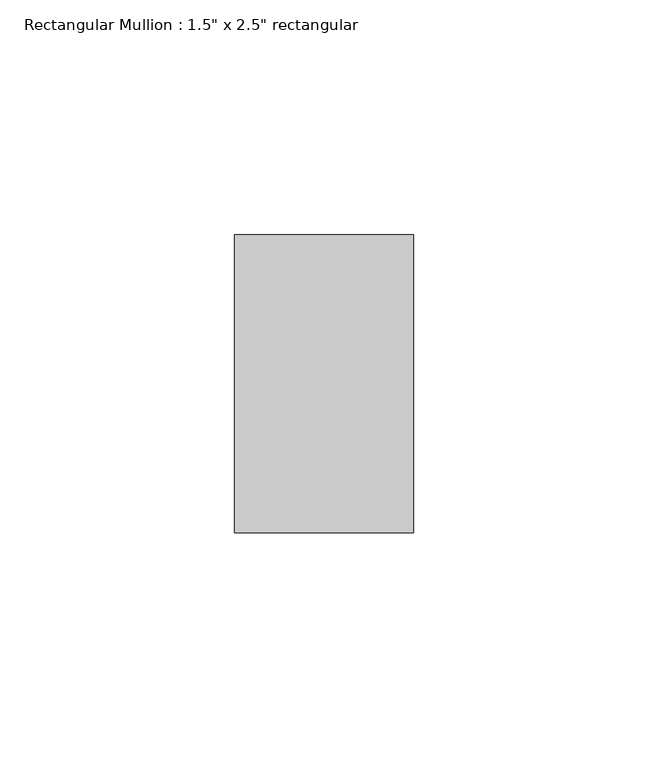
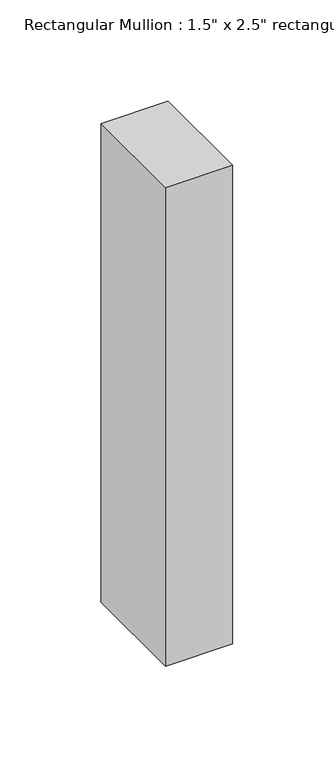
"""IFC4 building model written with IfcOpenShell, lengths in millimetres: member geometry."""

from ifc_helpers import new_model, si_unit, frame, origin, place, context, project, spatial, polyline, outline, extrude, source, transform, mapped, element, save


def member_00eacae2(model_context):
    return source(origin(), model_context, "Body", "SweptSolid", [
        extrude(outline(polyline([(19.05, 31.75), (19.05, -31.75), (-19.05, -31.75), (-19.05, 31.75), (19.05, 31.75)])), frame((0.0, 0.0, -288.2320668), z_axis=(0.0, 0.0, 1.0), x_axis=(1.0, 0.0, 0.0)), (0.0, 0.0, 1.0), 288.2320668),
    ])


if __name__ == "__main__":
    model = new_model("IFC4")
    model_context = context("Model", 3, world=origin())
    ifc_project = project(units=[si_unit("LENGTHUNIT", "METRE", prefix="MILLI")], contexts=[model_context])
    site = spatial("IfcSite", under=ifc_project)
    building = spatial("IfcBuilding", under=site)
    placement = place(None, origin())
    member_shape = member_00eacae2(model_context)
    element("IfcMember", 1, ObjectType="Rectangular Mullion : 1.5\" x 2.5\" rectangular", at=placement, inside=building, context=model_context, shape_type="MappedRepresentation", body=[
        mapped(member_shape, transform((0.0, 0.0, 0.0), x_axis=(1.0, 0.0, 0.0), y_axis=(0.0, 1.0, 0.0), z_axis=(0.0, 0.0, 1.0))),
    ])
    save(model, "model.ifc")

# Revit data of these elements
# Type "Rectangular Mullion : 1.5\" x 2.5\" rectangular"
#   built-in parameter 1007304 = 0.208333 (stored number, unit not read)
#   built-in parameter 1007301 = 0.0625 (stored number, unit not read)
#   built-in parameter 1007300 = 0.0625 (stored number, unit not read)
# Element 1 (IfcMember, "Rectangular Mullion : 1.5\" x 2.5\" rectangular")
#   Materials on its faces: "Aluminum"
# Materials
#   "Aluminum": class "Metal", colour RGB 247 247 247, transparency 0, Description = "Aluminum 6061", Cost = 0
